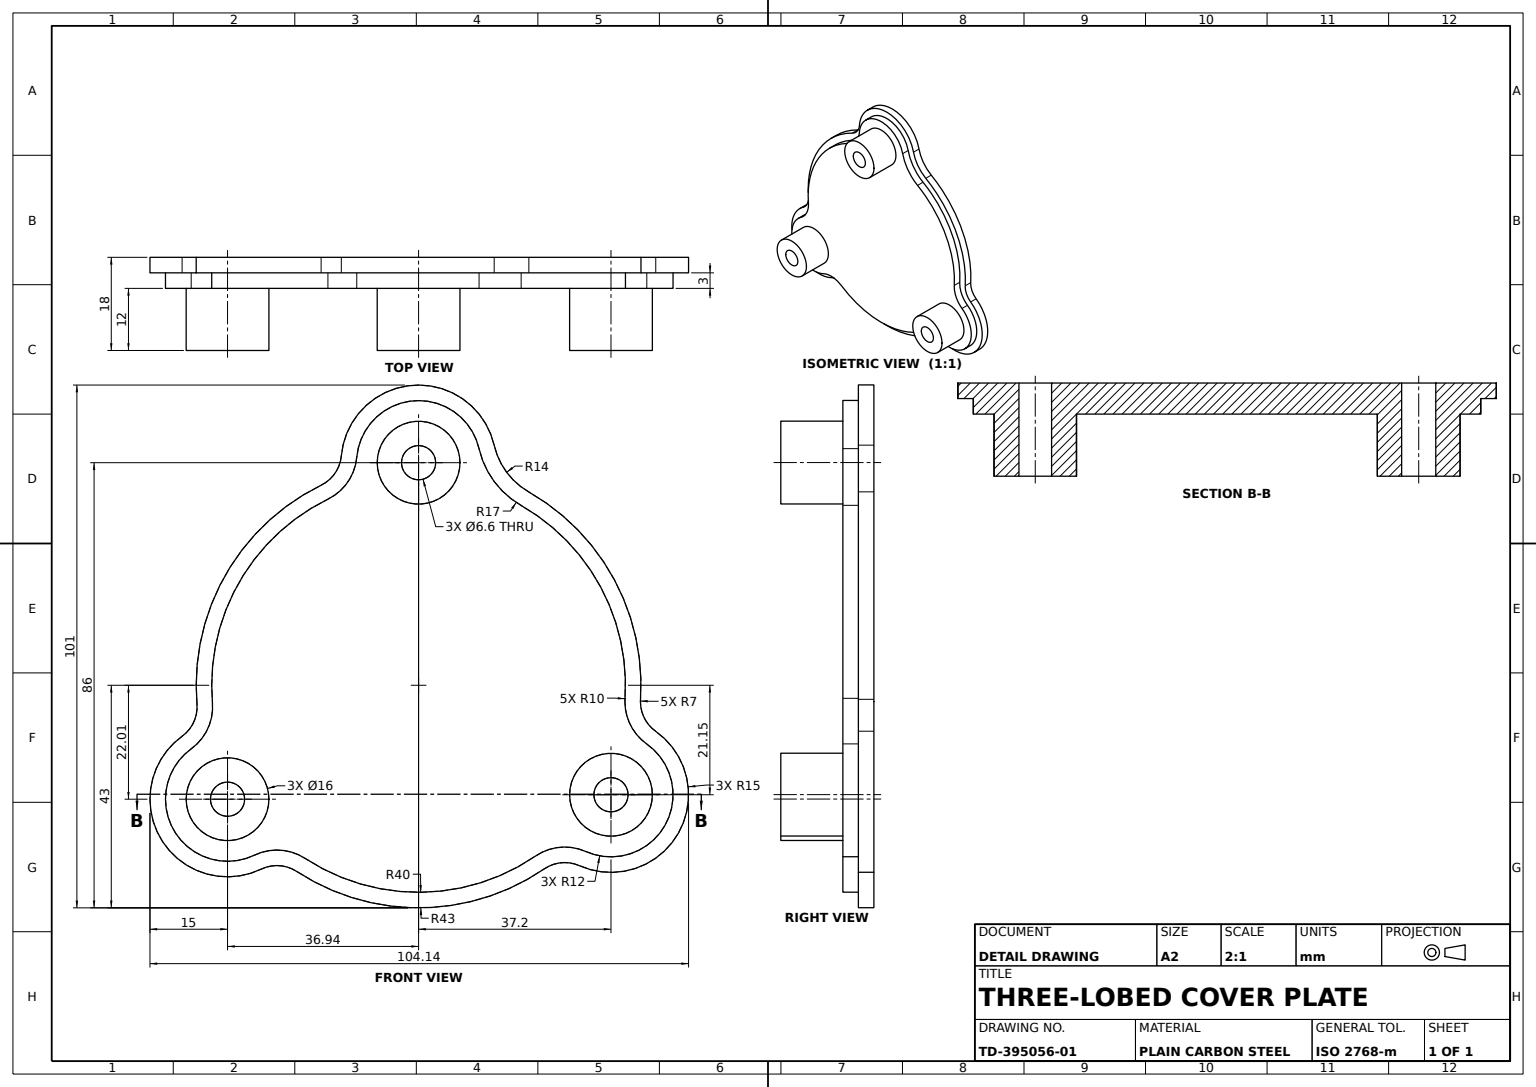
SolidWorks part; units mm, degrees
material "Plain Carbon Steel"
ref_plane "Front Plane" through (0, 0, 0) normal (0, 0, 1) x (1, 0, 0)
ref_plane "Top Plane" through (0, 0, 0) normal (0, 1, 0) x (1, 0, 0)
ref_plane "Right Plane" through (0, 0, 0) normal (1, 0, 0) x (0, 0, -1)
sketch "Base Plate Profile" plane through (0, 0, 0) normal (0, 0, 1) x (1, 0, 0)
  arc A0 (42.9127, -2.7392) -> (21.3206, 37.3421) centre (0, 0) ccw
  arc A1 (14.6184, 46.3621) -> (-14.9415, 44.324) centre (0, 43) ccw
  arc A2 (31.1024, -34.8558) -> (45.8589, -8.9019) centre (37.2028, -21.1523) ccw
  arc A3 (-45.7253, -9.8518) -> (-30.4296, -35.5233) centre (-36.9401, -22.0098) ccw
  arc A4 (14.6184, 46.3621) -> (21.3206, 37.3421) centre (28.2622, 49.5) ccw
  arc A5 (42.9127, -2.7392) -> (45.8589, -8.9019) centre (49.8985, -3.1851) ccw
  arc A6 (31.1024, -34.8558) -> (24.2998, -35.4756) centre (28.2556, -41.2507) ccw
  arc A7 (-45.7253, -9.8518) -> (-42.8496, -3.5931) centre (-49.8251, -4.178) ccw
  arc A8 (-18.8462, 38.65) -> (-14.9415, 44.324) centre (-21.9141, 44.9419) ccw
  arc A9 (-23.5566, -35.9734) -> (-30.4296, -35.5233) centre (-27.3914, -41.8296) ccw
  arc A10 (-23.5566, -35.9734) -> (24.2998, -35.4756) centre (0, 0) ccw
  arc A11 (-18.8462, 38.65) -> (-42.8496, -3.5931) centre (0, 0) ccw
  point P11 (17.0248, 41.1501)
  dimension "D1" = 86
  dimension "D2" = 30
  dimension "D3" = 30
  dimension "D4" = 30
  dimension "D8" = 14
  dimension "D9" = 14
  dimension "D10" = 7
  dimension "D11" = 14
  dimension "D12" = 14
  dimension "D13" = 14
  dimension "D5" = 22.0098
  dimension "D6" = 21.1523
  dimension "D7" = 37.2028
  dimension "D14" = 43
extrude "Base Plate" add sketch "Base Plate Profile" along normal blind 3
ref_plane "Plane1" through (0, 0, 3) normal (0, 0, 1) x (1, 0, 0)
sketch "Offset Step Profile" plane through (0, 0, 3) normal (0, 0, 1) x (1, 0, 0)
  arc A0 (-17.5313, 35.9535) -> (-39.8601, -3.3424) centre (0, 0) ccw
  arc A1 (-43.9683, -12.2834) -> (-39.8601, -3.3424) centre (-49.8251, -4.178) ccw
  arc A2 (-43.9683, -12.2834) -> (-31.7317, -32.8206) centre (-36.9401, -22.0098) ccw
  arc A3 (-21.9131, -33.4637) -> (-31.7317, -32.8206) centre (-27.3914, -41.8296) ccw
  arc A4 (-21.9131, -33.4637) -> (22.6045, -33.0006) centre (0, 0) ccw
  arc A5 (32.3225, -32.1151) -> (22.6045, -33.0006) centre (28.2556, -41.2507) ccw
  arc A6 (32.3225, -32.1151) -> (44.1277, -11.352) centre (37.2028, -21.1523) ccw
  arc A7 (39.9188, -2.5481) -> (44.1277, -11.352) centre (49.8985, -3.1851) ccw
  arc A8 (39.9188, -2.5481) -> (19.8331, 34.7368) centre (0, 0) ccw
  arc A9 (11.6947, 45.6897) -> (19.8331, 34.7368) centre (28.2622, 49.5) ccw
  arc A10 (11.6947, 45.6897) -> (-11.9532, 44.0592) centre (0, 43) ccw
  arc A11 (-17.5313, 35.9535) -> (-11.9532, 44.0592) centre (-21.9141, 44.9419) ccw
  arc A12 (-18.8462, 38.65) -> (-42.8496, -3.5931) centre (0, 0) ccw
  arc A13 (-45.7253, -9.8518) -> (-42.8496, -3.5931) centre (-49.8251, -4.178) ccw
  arc A14 (-45.7253, -9.8518) -> (-30.4296, -35.5233) centre (-36.9401, -22.0098) ccw
  arc A15 (-23.5566, -35.9734) -> (-30.4296, -35.5233) centre (-27.3914, -41.8296) ccw
  arc A16 (-23.5566, -35.9734) -> (24.2998, -35.4756) centre (0, 0) ccw
  arc A17 (31.1024, -34.8558) -> (24.2998, -35.4756) centre (28.2556, -41.2507) ccw
  arc A18 (31.1024, -34.8558) -> (45.8589, -8.9019) centre (37.2028, -21.1523) ccw
  arc A19 (42.9127, -2.7392) -> (45.8589, -8.9019) centre (49.8985, -3.1851) ccw
  arc A20 (42.9127, -2.7392) -> (21.3206, 37.3421) centre (0, 0) ccw
  arc A21 (14.6184, 46.3621) -> (21.3206, 37.3421) centre (28.2622, 49.5) ccw
  arc A22 (14.6184, 46.3621) -> (-14.9415, 44.324) centre (0, 43) ccw
  arc A23 (-18.8462, 38.65) -> (-14.9415, 44.324) centre (-21.9141, 44.9419) ccw
  arc A24 (-18.8462, 38.65) -> (-42.8496, -3.5931) centre (0, 0) ccw
  arc A25 (-45.7253, -9.8518) -> (-42.8496, -3.5931) centre (-49.8251, -4.178) ccw
  arc A26 (-45.7253, -9.8518) -> (-30.4296, -35.5233) centre (-36.9401, -22.0098) ccw
  arc A27 (-23.5566, -35.9734) -> (-30.4296, -35.5233) centre (-27.3914, -41.8296) ccw
  arc A28 (-23.5566, -35.9734) -> (24.2998, -35.4756) centre (0, 0) ccw
  arc A29 (31.1024, -34.8558) -> (24.2998, -35.4756) centre (28.2556, -41.2507) ccw
  arc A30 (31.1024, -34.8558) -> (45.8589, -8.9019) centre (37.2028, -21.1523) ccw
  arc A31 (42.9127, -2.7392) -> (45.8589, -8.9019) centre (49.8985, -3.1851) ccw
  arc A32 (42.9127, -2.7392) -> (21.3206, 37.3421) centre (0, 0) ccw
  arc A33 (14.6184, 46.3621) -> (21.3206, 37.3421) centre (28.2622, 49.5) ccw
  arc A34 (14.6184, 46.3621) -> (-14.9415, 44.324) centre (0, 43) ccw
  arc A35 (-18.8462, 38.65) -> (-14.9415, 44.324) centre (-21.9141, 44.9419) ccw
  dimension "D1" = 0
  dimension "D2" = 3
extrude "Offset Step" add sketch "Offset Step Profile" along normal blind 3 contours A0 A1 A2 A3 A4 A5 A6 A7 A8 A9 A10 A11
sketch "Standoff Boss Profile 3xØ16" plane through (0, 0, 6) normal (0, 0, 1) x (1, 0, 0)
  circle A0 centre (0, 43) radius 8
  circle A1 centre (37.2028, -21.1523) radius 8
  circle A2 centre (-36.9401, -22.0098) radius 8
  dimension "D1" = 16
  dimension "D2" = 16
  dimension "D3" = 16
extrude "Standoff Bosses 3xØ16" add sketch "Standoff Boss Profile 3xØ16" along normal blind 12
sketch "Mounting Hole Profile 3xØ6.6" plane through (0, 0, 18) normal (0, 0, 1) x (1, 0, 0)
  circle A0 centre (0, 43) radius 3.3
  circle A1 centre (37.2028, -21.1523) radius 3.3
  circle A2 centre (-36.9401, -22.0098) radius 3.3
  dimension "D1" = 6.6
  dimension "D2" = 6.6
  dimension "D3" = 6.6
extrude "Mounting Holes 3xØ6.6" cut sketch "Mounting Hole Profile 3xØ6.6" against normal blind 66
